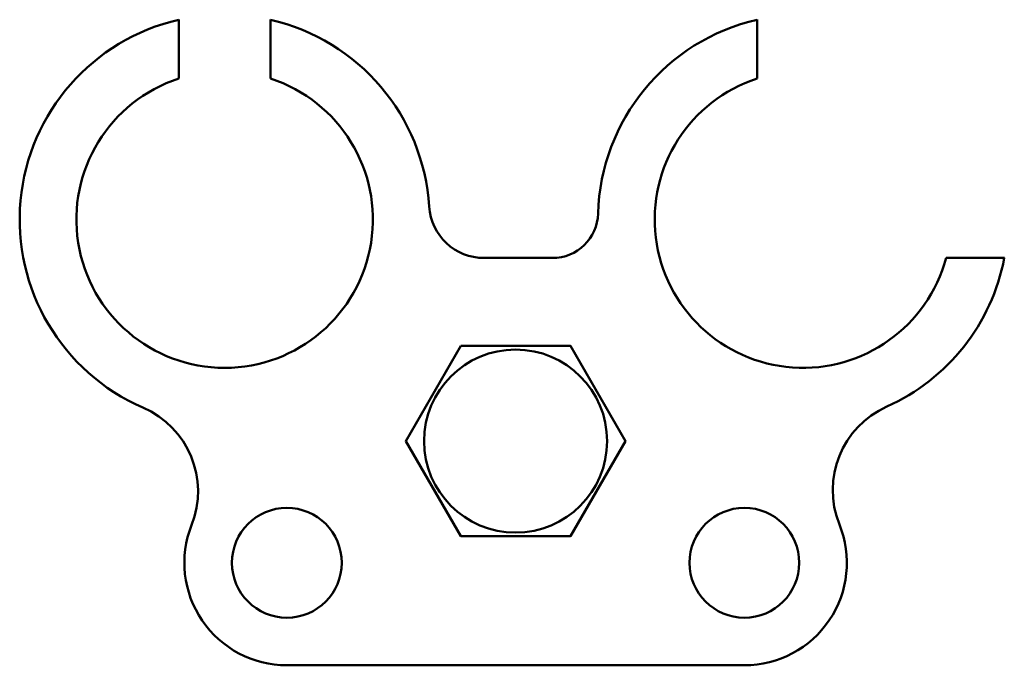
# Model space of a CAD drawing. Units: inches. Extents: x 1231 to 1339, y 671 to 741.
import ezdxf

# ---------------------------------------------------------------- set-up
doc = ezdxf.new("R2010")
doc.units = ezdxf.units.IN
doc.header["$MEASUREMENT"] = 0
doc.layers.add('M-OUTL', color=7, linetype='Continuous', lineweight=50)

msp = doc.modelspace()

# ---------------------------------------------------------------- linework, layer by layer
at = {"layer": 'M-OUTL'}
for p, q in [((1248.89, 741.04), (1248.89, 734.61)), ((1258.89, 741.04), (1258.89, 734.61)), ((1312.09, 741.04), (1312.09, 734.61)), ((1282.24, 715), (1289.71, 715)), ((1332.74, 715), (1339.1, 715)), ((1260.69, 670.5), (1310.69, 670.5))]:
    msp.add_line(p, q, dxfattribs=at)
at = {"layer": 'M-OUTL', "elevation": 5}
msp.add_lwpolyline([(1279.69, 705.39), (1273.69, 695), (1279.69, 684.61), (1291.69, 684.61), (1297.69, 695), (1291.69, 705.39)], close=True, dxfattribs=at)
at = {"layer": 'M-OUTL'}
for centre, radius in [((1285.69, 695, 5), 10), ((1260.69, 681.7), 6), ((1310.69, 681.7), 6)]:
    msp.add_circle(centre, radius, dxfattribs=at)
for centre, radius, start, end in [((1253.89, 719.2), 22.4, 102.8979, 246.5025), ((1253.89, 719.2), 22.4, 3.6339, 77.1021), ((1317.09, 719.2), 22.4, 102.8979, 178.3269), ((1253.89, 719.2), 16.2, 107.9774, 72.0226), ((1317.09, 719.2), 16.2, 107.9774, 344.9739), ((1282.24, 721), 6, 183.6339, 270), ((1289.71, 720), 5, 270, 358.3269), ((1317.09, 719.2), 22.4, 294.1549, 349.1931), ((1240.98, 689.49), 10, 338.451, 66.5025), ((1330.35, 689.64), 10, 114.1549, 201.986), ((1260.69, 681.7), 11.2, 158.451, 270), ((1310.69, 681.7), 11.2, 270, 21.986)]:
    msp.add_arc(centre, radius, start, end, dxfattribs=at)

doc.saveas('drawing.dxf')
